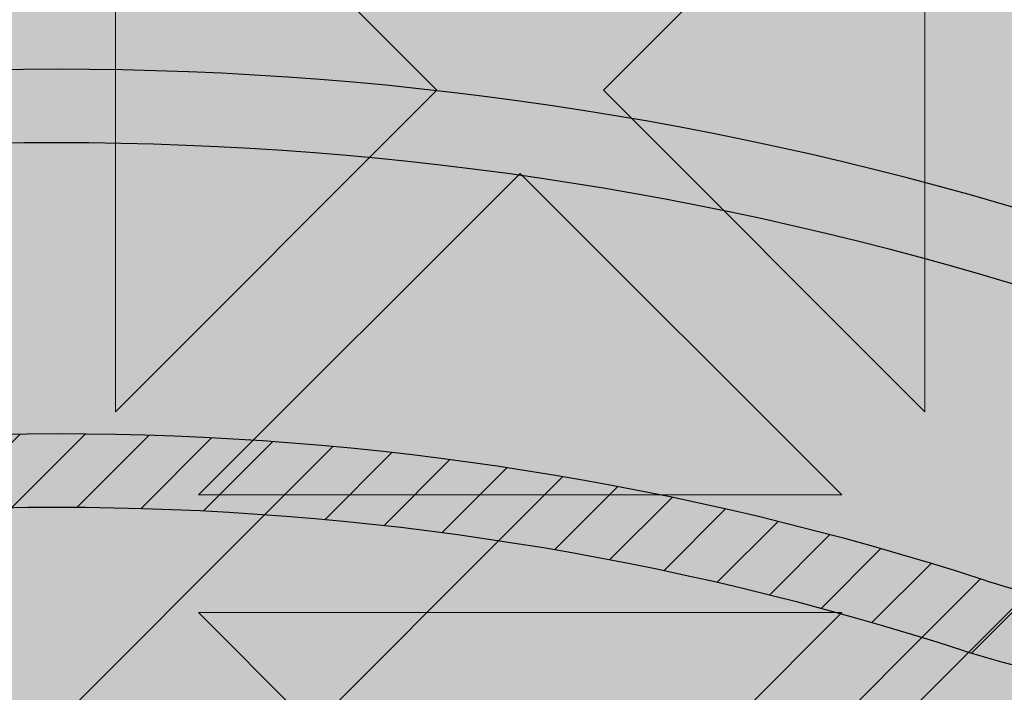
# Model space of a CAD drawing. Units: inches. Extents: x 844 to 2234, y 346 to 1084.
# Tile 20 of 93: x 1122.777 to 1124.911, y 703.603 to 705.06. Entities that reach past the tile are written whole.
import ezdxf

# ---------------------------------------------------------------- set-up
doc = ezdxf.new("R2010")
doc.units = ezdxf.units.IN
doc.header["$MEASUREMENT"] = 0
for name, color, linetype, lineweight in [('A-ANNO-DIMS', 2, 'Continuous', 18), ('furniture', 8, 'Continuous', 18), ('RA-AP-01$0$INT', 35, 'Continuous', 5)]:
    doc.layers.add(name, color=color, linetype=linetype, lineweight=lineweight)
doc.layers.add('RA-AP-01$0$FURN', color=3, linetype='Continuous')
doc.layers.add('RA-AP-01$0$WOOD', color=64, linetype='Continuous')
doc.styles.get("Standard").update_dxf_attribs({"font": 'arial.ttf'})
doc.dimstyles.get("Standard").update_dxf_attribs({"dimtxt": 6, "dimasz": 3, "dimexe": 0.18, "dimexo": 0.0625, "dimgap": 0.09, "dimtad": 0, "dimtih": 1, "dimtoh": 1, "dimdec": 1, "dimzin": 0, "dimdsep": 46, "dimlunit": 3, "dimtxsty": 'Standard', "dimblk": 'ARCHTICK', "dimcen": 0.09, "dimadec": 0, "dimazin": 0, "dimtfac": 1, "dimtdec": 1, "dimtofl": 0, "dimtmove": 0, "dimatfit": 3, "dimfxl": 1, "dimtolj": 1, "dimtzin": 0, "dimarcsym": 0})

# ---------------------------------------------------------------- blocks, each defined once
blk = doc.blocks.new('A$C18D01794')
at = {"layer": 'RA-AP-01$0$INT'}
h = blk.add_hatch(color=256, dxfattribs=at)
h.paths.add_polyline_path([(4.585917135068448, -7.856712009587804), (4.614201406330596, -7.856712009587056), (4.668846067270487, -7.802067348644738), (4.723490728212344, -7.856712009584164), (4.771774999457151, -7.856712009582887), (4.826419660396886, -7.80206734864072), (4.862780050090322, -7.838427738332541), (4.844495778842715, -7.856712009580965), (4.862780050090411, -7.856712009580482), (4.905206456960182, -7.814285602707865), (4.947632863832445, -7.856712009578238), (4.965917135079675, -7.856712009577755), (4.947632863831759, -7.838427738330656), (4.983993253523576, -7.802067348637219), (5.038637914464627, -7.856712009575829), (5.08692218571208, -7.856712009574554), (5.141566846649976, -7.802067348634224), (5.196211507589851, -7.856712009571666), (5.224495778822615, -7.856712009570916), (4.905206456953975, -7.537422687702283)])
h.paths.add_polyline_path([(4.895206456956031, -7.575706958950402), (4.895206456958921, -7.684996280828174), (4.840561796018589, -7.630351619890275)], flags=16)
h.paths.add_polyline_path([(4.915206456955638, -7.575706958949956), (4.969851117895509, -7.630351619887399), (4.915206456957609, -7.684996280827732)], flags=16)
h.paths.add_polyline_path([(4.826419660395175, -7.644493755514321), (4.881064321335613, -7.699138416452331), (4.771774999456703, -7.69913841645522)], flags=16)
h.paths.add_polyline_path([(4.983993253519558, -7.644493755510815), (5.038637914460456, -7.699138416449285), (4.929348592581548, -7.69913841645126)], flags=16)
h.paths.add_polyline_path([(4.881064321336025, -7.719138416452334), (4.826419660397532, -7.773783077393256), (4.771774999457062, -7.719138416455217)], flags=16)
h.paths.add_polyline_path([(4.929348592582019, -7.71913841645126), (5.038637914460982, -7.719138416449284), (4.983993253522945, -7.773783077389749)], flags=16)
h.paths.add_polyline_path([(4.895206456960191, -7.733280552075633), (4.895206456962115, -7.806001331460164), (4.876922185715016, -7.824285602708492), (4.840561796021581, -7.787925213016675)], flags=16)
h.paths.add_polyline_path([(4.915206456958487, -7.733280552075187), (4.969851117899527, -7.787925213013798), (4.933490728206909, -7.824285602708034), (4.9152064569598, -7.806001331461736)], flags=16)
h.paths.add_polyline_path([(4.757632863832376, -7.733280552079264), (4.812277524772842, -7.787925213017304), (4.757632863834348, -7.842569873958233)], flags=16)
h.paths.add_polyline_path([(4.737632863832376, -7.73328055207979), (4.737632863834348, -7.842569873958701), (4.682988202893906, -7.787925213020692)], flags=16)
h.paths.add_polyline_path([(5.05278005008503, -7.733280552072701), (5.052780050087917, -7.842569873951664), (4.998135389146995, -7.787925213013169)], flags=16)
h.paths.add_polyline_path([(5.072780050085024, -7.733280552072333), (5.127424711025931, -7.787925213010806), (5.072780050087916, -7.842569873951244)], flags=16)
h.paths.add_polyline_path([(4.935917135072783, -7.506712009583784), (5.255206456948811, -7.826001331459767), (5.255206456948932, -7.797717060211899), (5.200561796010279, -7.743072399273238), (5.255206456949403, -7.688427738334128), (5.25520645694961, -7.640143467086677), (5.200561796009787, -7.585498806146837), (5.236922185702417, -7.549138416454212), (5.255206456949919, -7.56742268770172), (5.255206456949998, -7.549138416454178), (5.212780050078687, -7.506712009583814), (5.25520645695036, -7.464285602712145), (5.255206456950438, -7.446001331464763), (5.236922185702424, -7.464285602712779), (5.200561796009796, -7.427925213020149), (5.255206456950753, -7.373280552079203), (5.25520645695096, -7.324996280834394), (5.200561796010322, -7.270351619893748), (5.255206456951428, -7.215706958952649), (5.255206456951547, -7.187422687705071)])
h.paths.add_polyline_path([(5.042988202883395, -7.42792521302065), (5.097632863823085, -7.373280552080975), (5.097632863822622, -7.482569873959883)], flags=16)
h.paths.add_polyline_path([(5.028846067259663, -7.442067348644384), (5.083490728198774, -7.496712009583504), (4.974201406321001, -7.496712009583035)], flags=16)
h.paths.add_polyline_path([(5.117632863823087, -7.37328055208089), (5.172277524762331, -7.42792521302015), (5.11763286382262, -7.482569873959851)], flags=16)
h.paths.add_polyline_path([(5.08349072819877, -7.516712009582191), (5.028846067259652, -7.571356670521302), (4.974201406320998, -7.516712009582638)], flags=16)
h.paths.add_polyline_path([(5.131774999446817, -7.35913841645716), (5.186419660386065, -7.413783077396415), (5.241064321325782, -7.359138416456712)], flags=17)
h.paths.add_polyline_path([(5.131774999446228, -7.496712009583703), (5.186419660386065, -7.442067348643883), (5.222780050079488, -7.478427738337313), (5.204495778832781, -7.496712009584014)], flags=16)
h.paths.add_polyline_path([(5.097632863822613, -7.530854145205813), (5.097632863823061, -7.640143467084723), (5.042988202883383, -7.585498806145032)], flags=16)
h.paths.add_polyline_path([(5.131774999446899, -7.339138416457162), (5.241064321325809, -7.339138416456712), (5.186419660386591, -7.284493755517479)], flags=17)
h.paths.add_polyline_path([(5.131774999446226, -7.516712009581999), (5.204495778830767, -7.516712009581702), (5.22278005007868, -7.534996280829206), (5.186419660386049, -7.571356670521828)], flags=16)
h.paths.add_polyline_path([(5.11763286382262, -7.530854145205852), (5.17227752476232, -7.585498806145562), (5.117632863823064, -7.64014346708481)], flags=16)
h.paths.add_polyline_path([(5.186419660386069, -7.599640941770585), (5.241064321325754, -7.654285602710281), (5.131774999446791, -7.654285602709814)], flags=16)
h.paths.add_polyline_path([(5.131774999446872, -7.674285602709813), (5.24106432132578, -7.674285602710282), (5.186419660386554, -7.728930263649504)], flags=16)
h.paths.add_polyline_path([(5.255206456951811, -7.126001331467467), (5.255206456951895, -7.106712009588038), (4.555206456956052, -7.106712009588038), (4.555206456956136, -7.12600133146746), (4.905206456953973, -7.476001331465289)])
h.paths.add_polyline_path([(4.983993253513404, -7.368930263651977), (4.92934859257295, -7.314285602713969), (5.03863791445186, -7.314285602711063)], flags=16)
h.paths.add_polyline_path([(4.969851117889988, -7.383072399276016), (4.915206456952556, -7.437717060215906), (4.915206456949648, -7.328427738338133)], flags=16)
h.paths.add_polyline_path([(4.929348592572535, -7.294285602713971), (4.983993253511019, -7.239640941773039), (5.038637914451496, -7.294285602711065)], flags=16)
h.paths.add_polyline_path([(5.052780050074912, -7.280143467087016), (4.998135389134438, -7.225498806148989), (5.052780050072919, -7.170854145208052)], flags=16)
h.paths.add_polyline_path([(5.07278005007491, -7.280143467086489), (5.072780050072918, -7.170854145207579), (5.127424711013374, -7.225498806145578)], flags=16)
h.paths.add_polyline_path([(4.89520645695295, -7.437717060216355), (4.840561796013067, -7.383072399278919), (4.895206456950961, -7.328427738338582)], flags=16)
h.paths.add_polyline_path([(4.915206456948365, -7.280143467090674), (4.915206456946434, -7.207422687704125), (4.933490728192729, -7.18913841645701), (4.969851117886972, -7.225498806149623)], flags=16)
h.paths.add_polyline_path([(4.881064321327021, -7.314285602715054), (4.82641966038902, -7.368930263655506), (4.771774999448108, -7.314285602717047)], flags=16)
h.paths.add_polyline_path([(4.895206456950073, -7.280143467091125), (4.840561796009022, -7.225498806152518), (4.876922185700835, -7.18913841645908), (4.895206456948749, -7.207422687706589)], flags=16)
h.paths.add_polyline_path([(4.983993253510392, -7.211356670525576), (4.947632863816944, -7.174996280833758), (4.965917135064043, -7.156712009585847), (5.038637914448995, -7.156712009584522)], flags=16)
h.paths.add_polyline_path([(4.881064321326543, -7.294285602715056), (4.771774999447578, -7.294285602717046), (4.826419660385607, -7.239640941776569)], flags=16)
h.paths.add_polyline_path([(4.905206456946447, -7.19913841645844), (4.862780050074785, -7.156712009587725), (4.947632863816685, -7.156712009586302)], flags=16)
h.paths.add_polyline_path([(5.14156684663679, -7.211356670521528), (5.086922185696452, -7.156712009583639), (5.196211507574223, -7.156712009581651)], flags=16)
h.paths.add_polyline_path([(4.8264196603837, -7.211356670529104), (4.771774999442643, -7.156712009590501), (4.8444957788276, -7.156712009588568), (4.862780050075511, -7.17499628083566)], flags=16)
h.paths.add_polyline_path([(4.812277524760289, -7.225498806153156), (4.757632863822258, -7.28014346709363), (4.757632863819352, -7.170854145214669)], flags=16)
h.paths.add_polyline_path([(4.73763286382226, -7.280143467093997), (4.682988202881349, -7.22549880615554), (4.737632863819352, -7.170854145215086)], flags=16)
h.paths.add_polyline_path([(4.723490728195188, -7.156712009591787), (4.668846067257299, -7.211356670532127), (4.614201406317417, -7.156712009594693)], flags=16)
h.paths.add_polyline_path([(4.597632863829262, -7.506712009583814), (4.555206456957951, -7.54913841645418), (4.555206456958029, -7.56742268770172), (4.573490728205535, -7.549138416454212), (4.609851117898167, -7.585498806146839), (4.555206456958338, -7.640143467086675), (4.555206456958546, -7.688427738334125), (4.60985111789767, -7.743072399273238), (4.555206456959015, -7.797717060211899), (4.555206456959138, -7.826001331459767), (4.874495778835167, -7.506712009583786), (4.5552064569564, -7.187422687705062), (4.555206456956523, -7.215706958952644), (4.609851117897629, -7.270351619893746), (4.555206456956988, -7.324996280834396), (4.555206456957198, -7.373280552079195), (4.609851117898153, -7.427925213020147), (4.573490728205528, -7.464285602712779), (4.555206456957507, -7.446001331464756), (4.555206456957585, -7.464285602712143)])
h.paths.add_polyline_path([(4.712780050085332, -7.482569873959882), (4.712780050084863, -7.373280552080972), (4.767424711024555, -7.42792521302065)], flags=16)
h.paths.add_polyline_path([(4.726922185709173, -7.496712009583504), (4.781566846648288, -7.442067348644384), (4.836211507586949, -7.496712009583033)], flags=16)
h.paths.add_polyline_path([(4.692780050085327, -7.482569873959851), (4.638135389145619, -7.427925213020149), (4.692780050084865, -7.373280552080892)], flags=16)
h.paths.add_polyline_path([(4.726922185709182, -7.516712009582191), (4.836211507586949, -7.51671200958264), (4.7815668466483, -7.571356670521304)], flags=16)
h.paths.add_polyline_path([(4.678637914461726, -7.496712009583706), (4.605917135075169, -7.496712009584014), (4.587632863828464, -7.478427738337311), (4.623993253521887, -7.442067348643881)], flags=16)
h.paths.add_polyline_path([(4.712780050085336, -7.530854145205816), (4.767424711024568, -7.585498806145034), (4.71278005008489, -7.640143467084724)], flags=16)
h.paths.add_polyline_path([(4.678637914461726, -7.516712009582001), (4.623993253521899, -7.571356670521829), (4.587632863829271, -7.534996280829206), (4.605917135077185, -7.5167120095817)], flags=16)
h.paths.add_polyline_path([(4.692780050085336, -7.530854145205848), (4.692780050084889, -7.64014346708481), (4.638135389145632, -7.585498806145562)], flags=16)
h.paths.add_polyline_path([(4.623993253521885, -7.413783077396415), (4.678637914461131, -7.359138416457161), (4.56934859258217, -7.359138416456712)], flags=17)
h.paths.add_polyline_path([(4.623993253521901, -7.599640941770568), (4.678637914461158, -7.654285602709814), (4.569348592582195, -7.654285602710281)], flags=16)
h.paths.add_polyline_path([(4.678637914461051, -7.339138416457162), (4.623993253521361, -7.284493755517479), (4.569348592582143, -7.339138416456712)], flags=17)
h.paths.add_polyline_path([(4.678637914461076, -7.674285602709813), (4.623993253521399, -7.728930263649504), (4.569348592582167, -7.674285602710281)], flags=16)
h = blk.add_hatch(color=256, dxfattribs=at)
h.paths.add_polyline_path([(4.905206456954232, -7.537422687702028), (4.874495778835232, -7.506712009583718), (4.555206456959138, -7.826001331459766), (4.555206456959269, -7.856712009588616), (4.585917135068449, -7.856712009587804)])
h.paths.add_polyline_path([(4.935917135072152, -7.506712009583152), (4.905206456953497, -7.537422687701806), (5.224495778822614, -7.856712009570917), (5.255206456948681, -7.856712009570104), (5.255206456948813, -7.826001331459768)])
h.paths.add_polyline_path([(5.255206456951549, -7.18742268770507), (5.255206456951813, -7.126001331467461), (4.905206456953563, -7.476001331465701), (4.935917135072559, -7.506712009584006)])
h.paths.add_polyline_path([(4.874495778835167, -7.506712009583785), (4.905206456953818, -7.476001331465132), (4.555206456956135, -7.126001331467458), (4.555206456956399, -7.187422687705064)])
h = blk.add_hatch(color=256, dxfattribs=at)
h.paths.add_polyline_path([(4.969851117891331, -7.630351619889621), (4.915206456952669, -7.575706958950966), (4.915206456952222, -7.684996280828739)])
h.paths.add_polyline_path([(4.895206456953064, -7.575706958950968), (4.840561796014413, -7.630351619889628), (4.895206456953533, -7.684996280828741)])
h.paths.add_polyline_path([(4.826419660390684, -7.644493755513362), (4.771774999451003, -7.699138416453052), (4.881064321329913, -7.699138416452587)])
h.paths.add_polyline_path([(4.881064321329884, -7.719138416452585), (4.771774999450921, -7.719138416453052), (4.82641966039018, -7.773783077392298)])
h.paths.add_polyline_path([(4.895206456953734, -7.733280552076196), (4.840561796013912, -7.787925213016031), (4.876922185707337, -7.824285602709455), (4.895206456954043, -7.806001331462747)])
h.paths.add_polyline_path([(4.862780050082808, -7.838427738332388), (4.826419660390178, -7.802067348639763), (4.771774999450351, -7.856712009579595), (4.844495778835303, -7.856712009579895)])
h.paths.add_polyline_path([(4.812277524766446, -7.787925213016036), (4.757632863827191, -7.733280552076788), (4.757632863826741, -7.842569873955747)])
h.paths.add_polyline_path([(4.737632863827191, -7.733280552076863), (4.682988202887508, -7.787925213016558), (4.737632863826743, -7.842569873955778)])
h.paths.add_polyline_path([(4.668846067263777, -7.802067348640287), (4.614201406325123, -7.856712009578949), (4.723490728202894, -7.856712009579402)])
h.paths.add_polyline_path([(4.905206456953846, -7.814285602708654), (4.862780050082654, -7.856712009579847), (4.947632863824561, -7.85671200958032)])
h.paths.add_polyline_path([(4.915206456952028, -7.733280552076195), (4.91520645695173, -7.806001331460731), (4.933490728199234, -7.824285602708648), (4.96985111789186, -7.787925213016022)])
h.paths.add_polyline_path([(5.038637914454841, -7.719138416453029), (4.929348592575874, -7.71913841645258), (4.983993253515593, -7.773783077392289)])
h.paths.add_polyline_path([(4.983993253515065, -7.644493755513352), (4.929348592575849, -7.699138416452582), (5.038637914454755, -7.699138416453031)])
h.paths.add_polyline_path([(5.052780050079843, -7.73328055207676), (4.998135389140595, -7.787925213016018), (5.052780050080309, -7.842569873955721)])
h.paths.add_polyline_path([(4.983993253516868, -7.802067348639752), (4.947632863824241, -7.838427738332383), (4.965917135071747, -7.856712009579888), (5.038637914456701, -7.856712009579572)])
h.paths.add_polyline_path([(5.127424711019533, -7.787925213016519), (5.072780050079843, -7.733280552076838), (5.07278005008031, -7.842569873955751)])
h.paths.add_polyline_path([(5.141566846643269, -7.802067348640248), (5.086922185704154, -7.85671200957937), (5.196211507581929, -7.856712009578901)])
for p, q in [((4.905206456953975, -7.537422687702283), (5.224495778822613, -7.856712009570916)), ((4.929348592581546, -7.69913841645126), (4.983993253519556, -7.644493755510815)), ((4.983993253519558, -7.644493755510817), (5.038637914460456, -7.699138416449285)), ((5.038637914460456, -7.699138416449285), (4.929348592581546, -7.69913841645126)), ((5.038637914460983, -7.719138416449284), (4.92934859258202, -7.71913841645126)), ((4.92934859258202, -7.71913841645126), (4.983993253522945, -7.773783077389751)), ((5.038637914460983, -7.719138416449284), (4.983993253522945, -7.773783077389751)), ((4.9152064569598, -7.806001331460137), (4.915206456958485, -7.733280552075186)), ((4.915206456958485, -7.733280552075186), (4.969851117899529, -7.787925213013799)), ((5.052780050085028, -7.733280552072701), (4.998135389146995, -7.787925213013169)), ((5.052780050085028, -7.733280552072701), (5.052780050087917, -7.842569873951664)), ((4.969851117899529, -7.787925213013798), (4.93349072820771, -7.824285602707234)), ((5.052780050087917, -7.842569873951664), (4.998135389146995, -7.787925213013169))]:
    blk.add_line(p, q, dxfattribs=at)
blk = doc.blocks.new('A$C32926AE1')
at = {"layer": 'RA-AP-01$0$WOOD'}
h = blk.add_hatch(color=256, dxfattribs=at)
h.dxf.hatch_style = 1
h.paths.add_polyline_path([(5.157430609644524, 4.573483066760929, -0.1009492694046607), (5.155401577623758, 4.593365984175333, -0.1842662638101597), (5.172249623284174, 4.638795604568598, 0.2056608120311276), (5.179560981299304, 4.661316324430096, 0.3614336704623542), (5.134352340494423, 4.706524965234944, 0.2056608120311297), (5.111831620632933, 4.699213607219793, -0.1842662638101113), (5.066402000239693, 4.682365561559342, -0.1055311479399994), (5.045656153913092, 4.68467289944697, 0.1567636581983829), (4.763886414745334, 4.684672899446966, -0.1055311479399895), (4.743140568418733, 4.68236556155934, -0.1842662638100833), (4.6977109480255, 4.69921360721979, 0.2056608120302612), (4.675190228164109, 4.706524965234949, 0.3614336704708441), (4.629981587358889, 4.66131632442871, 0.2056608120245944), (4.637292945374126, 4.638795604567974, -0.1842662638101024), (4.654140991034615, 4.59336598417475, -0.1009492694055169), (4.652111959013835, 4.573483066760181, 0.021410119221476), (4.629748025606143, 4.156712009541676, 0.0214101192214795), (4.652111959013809, 3.739940952323101, -0.1009492694059586), (4.654140991034615, 3.720058034908448, -0.1842662638100975), (4.637292945374126, 3.674628414515226, 0.2056608120245705), (4.629981587358889, 3.652107694654492, 0.3614336704708879), (4.675190228164113, 3.606899053848249, 0.2056608120302384), (4.697710948025501, 3.614210411863408, -0.1842662638100995), (4.743140568418738, 3.63105845752386, -0.1055311479402541), (4.763886414745388, 3.628751119636215, 0.1567636581983776), (5.045656153913137, 3.628751119636244, -0.1055311479397538), (5.066402000239692, 3.631058457523857, -0.1842662638101067), (5.111831620632931, 3.614210411863407, 0.2056608120310924), (5.134352340494417, 3.606899053848256, 0.3614336704624001), (5.179560981299307, 3.652107694653103, 0.2056608120311314), (5.172249623284175, 3.6746284145146, -0.1842662638101402), (5.155401577623758, 3.72005803490786, -0.1009492694051366), (5.15743060964455, 3.739940952322354, 0.0214101192215073), (5.179794543052287, 4.156712009541468, 0.0214101192215252)])
h.paths.add_polyline_path([(4.639748609479751, 4.156712009541513, 0.0213537860821624), (4.661970494867118, 3.741887061152232, -0.094075836301374), (4.664143710413708, 3.7196126951003, -0.1824818158568985), (4.644813765429836, 3.668037719127816, 0.2056608120245319), (4.639939526753007, 3.653023905887301, 0.3614336704710246), (4.676106439397173, 3.616856993242342, 0.2056608120302234), (4.691120252638095, 3.621731231919122, -0.1824818158602558), (4.742695228611606, 3.641061176902986, -0.1029891339458722), (4.766991894714349, 3.638256818950944, 0.156709409989566), (5.042550673941472, 3.638256818950105, -0.102989133958497), (5.066847340047078, 3.641061176902949, -0.1824818158594995), (5.118422316020358, 3.621731231919103, 0.2056608120311416), (5.133436129261316, 3.616856993242346, 0.3614336704621468), (5.169603041905217, 3.653023905886178, 0.2056608120310986), (5.164728803228477, 3.668037719127177, -0.1824818158565612), (5.145398858244737, 3.719612695099578, -0.0940758363009313), (5.147572073791232, 3.741887061151398, 0.0213537860822023), (5.169793959178681, 4.156712009541451, 0.0213537860822226), (5.147572073791203, 4.571536957931898, -0.0940758363005034), (5.145398858244737, 4.59381132398362, -0.1824818158565587), (5.164728803228476, 4.645386299956021, 0.2056608120311045), (5.169603041905216, 4.66040011319702, 0.3614336704621845), (5.133436129261313, 4.696567025840856, 0.2056608120310773), (5.118422316020359, 4.691692787164098, -0.182481815859508), (5.066847340047078, 4.67236284218025, -0.1029891339584606), (5.04255067394148, 4.675167200133092, 0.156709409989566), (4.766991894714357, 4.675167200132257, -0.1029891339458842), (4.742695228611611, 4.672362842180213, -0.1824818158602725), (4.691120252638095, 4.691692787164077, 0.2056608120302152), (4.676106439397174, 4.696567025840858, 0.3614336704710363), (4.639939526753005, 4.660400113195899, 0.2056608120245495), (4.644813765429837, 4.645386299955384, -0.1824818158568934), (4.664143710413708, 4.593811323982902, -0.0940758363009187), (4.661970494867149, 4.571536957931074, 0.021353786082177)], flags=16)
h.paths.add_polyline_path([(5.129794543052235, 4.432167055276933, -0.0141661062790638), (5.130152669293814, 4.156927903047693, -0.0141661062790647), (5.129794543052234, 3.881688750818433, -0.0785247771143638), (5.10979738006795, 3.755143611847103, 0.0945969212073497), (5.105408519571111, 3.717898134952927, 0.1043170707844957), (5.116074640131521, 3.670385395016088, 0.1043170707864965), (5.068561900193738, 3.681051515576561, 0.09459692119553), (5.031316423304057, 3.676662655080835, -0.1580239521427272), (4.778226145355827, 3.676662655080367, 0.0945969211986668), (4.740980668464973, 3.681051515576592, 0.1043170707882822), (4.693467928526415, 3.670385395015844, 0.1043170707867916), (4.704134049087309, 3.717898134953662, 0.0945969211972894), (4.69974518859162, 3.755143611844042, -0.0785247771163196), (4.679748025606343, 3.881688750818406, -0.0141661062790663), (4.679389899364763, 4.156927903047693, -0.0141661062790672), (4.679748025606343, 4.432167055276998, -0.0785247771163064), (4.699745188591625, 4.55871219425134, 0.094596921197333), (4.704134049087308, 4.595957671141738, 0.1043170707867205), (4.693467928526416, 4.643470411079523, 0.1043170707882628), (4.740980668464965, 4.632804290518776, 0.0945969211988114), (4.778226145355874, 4.637193151015016, -0.158023952142669), (5.031316423304015, 4.637193151014546, 0.0945969211956361), (5.068561900193736, 4.632804290518806, 0.1043170707864979), (5.11607464013152, 4.643470411079278, 0.1043170707844617), (5.105408519571112, 4.595957671142455, 0.0945969212074597), (5.109797380067959, 4.558712194248236, -0.0785247771143467)], flags=0)
h.paths.add_polyline_path([(5.119794532311105, 4.432259799204851, -0.0142000800617244), (5.120156169157484, 4.156927903047701, -0.0142000800617277), (5.119794532311105, 3.881596006890482, -0.0784894509520253), (5.100273383573699, 3.758192358677797, 0.0940138827242913), (5.095413455884425, 3.717477693979438, 0.0606271852308753), (5.099615656341024, 3.686844378806616, 0.0606271852322524), (5.068982341167493, 3.691046579263239, 0.0940138827010453), (5.028267676478798, 3.686186651576848, -0.1580706864508061), (4.781274892180912, 3.686186651576435, 0.0940138827026903), (4.740560227491556, 3.691046579263279, 0.0606271852339895), (4.709926912317155, 3.686844378806508, 0.0606271852329405), (4.714129112773991, 3.717477693980356, 0.094013882701304), (4.709269185087677, 3.758192358669163, -0.0784894509577193), (4.689748036347473, 3.881596006890469, -0.014200080061729), (4.689386399501094, 4.156927903047709, -0.0142000800617217), (4.689748036347473, 4.432259799204808, -0.078489450957724), (4.709269185087651, 4.555663447426125, 0.0940138827014585), (4.714129112773992, 4.596378112114996, 0.0606271852329731), (4.709926912317154, 4.62701142728886, 0.0606271852340196), (4.74056022749157, 4.622809226832087, 0.0940138827024997), (4.781274892180847, 4.627669154518912, -0.1580706864508359), (5.028267676478777, 4.627669154518526, 0.0940138827010946), (5.068982341167492, 4.622809226832129, 0.060627185232254), (5.099615656341024, 4.627011427288751, 0.0606271852308727), (5.095413455884425, 4.59637811211593, 0.0940138827241088), (5.100273383573675, 4.555663447417647, -0.0784894509520978)], flags=0)
h.paths.add_polyline_path([(5.06978912287499, 4.430218106756144, -0.014241683694547), (5.070173729147532, 4.156927903047672, -0.0142416836945458), (5.06978912287499, 3.883637699339223, -0.0800609523125196), (5.052662118612511, 3.773463122773442, 0.0526421978001116), (5.04590916754064, 3.740550867606997, 0.0526421977992423), (5.012996912374707, 3.73379791653534, -0.1583028414718258), (4.796545656286308, 3.73379791653451, 0.0526421978034211), (4.763633401117837, 3.740550867607021, 0.0526421978018622), (4.756880450045755, 3.773463122774558, -0.0800609523117106), (4.739753445783639, 3.883637699339268, -0.0142416836945435), (4.739368839511098, 4.156927903047671, -0.0142416836945477), (4.739753445783639, 4.430218106756155, -0.0800609523116345), (4.75688045004574, 4.540392683320762, 0.052642197801941), (4.763633401117837, 4.573304938488346, 0.0526421978035071), (4.796545656286361, 4.580057889560873, -0.1583028414717561), (5.012996912374669, 4.580057889560039, 0.0526421977993048), (5.04590916754064, 4.57330493848837, 0.0526421978002057), (5.052662118612529, 4.540392683321868, -0.080060952312477)], flags=0)
h.paths.add_polyline_path([(5.049789715110557, 4.43038092723357, -0.0143097550741839), (5.05018085590259, 4.156927903047715, -0.0143097550741854), (5.049789715110558, 3.883474878861827, -0.0800685599149176), (5.03362098255317, 3.779581877367999, 0.0306258898956367), (5.028241146483733, 3.758218888663947, 0.0306258898977031), (5.006878157778253, 3.75283905259408, -0.1583983521624096), (4.802664410878162, 3.752839052594731, 0.0306258898946014), (4.781301422174808, 3.758218888663924, 0.0306258898967912), (4.775921586105202, 3.779581877368794, -0.080068559914251), (4.759752853548071, 3.883474878861786, -0.0143097550741854), (4.759361712756037, 4.156927903047671, -0.0143097550741854), (4.759752853548071, 4.430380927233557, -0.0800685599142479), (4.775921586105193, 4.534273928726546, 0.0306258898968306), (4.781301422174808, 4.555636917431444, 0.0306258898945754), (4.802664410878143, 4.561016753500631, -0.1583983521624168), (5.006878157778244, 4.561016753501291, 0.0306258898977177), (5.028241146483733, 4.555636917431421, 0.0306258898958182), (5.03362098255321, 4.534273928727244, -0.080068559914796)], flags=0)
h.paths.add_polyline_path([(4.999766070382627, 4.428171244713864, -0.0143443147609634), (5.000198441819402, 4.156927903047689, -0.0143443147609612), (4.999766070382627, 3.885684561381556, -0.0784641635803329), (4.987356730658798, 3.799103304488872, -0.1506053783831347), (4.822185837999821, 3.79910330448882, -0.0784641635803318), (4.809776498276007, 3.885684561381509, -0.014344314760963), (4.809344126839227, 4.156927903047677, -0.0143443147609645), (4.809776498276007, 4.428171244713873, -0.0784641635803192), (4.822185837999822, 4.514752501606549, -0.1506053783831338), (4.987356730658798, 4.514752501606494, -0.078464163580285)], flags=0)
h.paths.add_polyline_path([(4.979755254238824, 4.42764379880488, -0.0143772539198268), (4.980205517789977, 4.156927903047693, -0.0143772539198275), (4.979755254238824, 3.886212007290489, -0.0689242507424422), (4.971183264704897, 3.815276770442801, -0.1296645318904179), (4.838359303953726, 3.815276770442746, -0.0689242507424186), (4.829787314419809, 3.886212007290419, -0.0143772539198292), (4.829337050868653, 4.156927903047653, -0.0143772539198325), (4.829787314419809, 4.427643798804946, -0.0689242507424211), (4.838359303953725, 4.498579035652621, -0.1296645318904187), (4.971183264704897, 4.498579035652565, -0.0689242507424401)], flags=0)
h = blk.add_hatch(color=256, dxfattribs=at)
h.dxf.hatch_style = 1
h.paths.add_polyline_path([(5.145398858244737, 4.59381132398362, -0.1824818158565616), (5.164728803228476, 4.645386299956021, 0.2056608120311045), (5.169603041905216, 4.66040011319702, 0.3614336704621845), (5.133436129261313, 4.696567025840856, 0.2056608120310773), (5.118422316020359, 4.691692787164098, -0.182481815859508), (5.066847340047078, 4.67236284218025, -0.1029891339584606), (5.04255067394148, 4.675167200133092, 0.156709409989566), (4.766991894714357, 4.675167200132257, -0.1029891339458842), (4.742695228611611, 4.672362842180213, -0.1824818158602725), (4.691120252638095, 4.691692787164077, 0.2056608120302152), (4.676106439397174, 4.696567025840858, 0.3614336704710363), (4.639939526753005, 4.660400113195899, 0.2056608120245495), (4.644813765429837, 4.645386299955384, -0.1824818158568934), (4.664143710413708, 4.593811323982902, -0.0940758363009187), (4.661970494867149, 4.571536957931074, 0.0213537860821772), (4.639748609479751, 4.156712009541507, 0.0213537860821625), (4.661970494867119, 3.741887061152226, -0.0940758363013071), (4.664143710413708, 3.719612695100309, -0.1824818158569294), (4.644813765429836, 3.668037719127816, 0.2056608120245319), (4.639939526753007, 3.653023905887301, 0.3614336704710246), (4.676106439397173, 3.616856993242342, 0.2056608120302234), (4.691120252638095, 3.621731231919122, -0.1824818158602558), (4.742695228611606, 3.641061176902986, -0.1029891339458722), (4.766991894714349, 3.638256818950944, 0.156709409989566), (5.042550673941472, 3.638256818950105, -0.102989133958497), (5.066847340047078, 3.641061176902949, -0.1824818158594995), (5.118422316020358, 3.621731231919103, 0.2056608120311416), (5.133436129261316, 3.616856993242346, 0.3614336704621468), (5.169603041905217, 3.653023905886178, 0.2056608120310986), (5.164728803228477, 3.668037719127177, -0.1824818158565612), (5.145398858244737, 3.719612695099578, -0.0940758363009313), (5.147572073791232, 3.741887061151398, 0.0213537860822023), (5.169793959178681, 4.156712009541451, 0.0213537860822226), (5.147572073791203, 4.571536957931898, -0.0940758363004996)])
h.paths.add_polyline_path([(5.109797380067958, 4.55871219424824, -0.0785247771143472), (5.129794543052234, 4.432167055276936, -0.0141661062790644), (5.130152669293814, 4.156927903047685, -0.014166106279066), (5.129794543052234, 3.881688750818401, -0.0785247771143517), (5.109797380067946, 3.755143611847092, 0.0945969212073132), (5.105408519571111, 3.717898134952929, 0.1043170707844995), (5.116074640131521, 3.670385395016088, 0.1043170707864965), (5.068561900193738, 3.681051515576561, 0.09459692119553), (5.031316423304057, 3.676662655080835, -0.1580239521427272), (4.778226145355827, 3.676662655080367, 0.0945969211986668), (4.740980668464973, 3.681051515576592, 0.1043170707882822), (4.693467928526415, 3.670385395015844, 0.1043170707867916), (4.704134049087309, 3.717898134953662, 0.0945969211972894), (4.69974518859162, 3.755143611844042, -0.0785247771163196), (4.679748025606343, 3.881688750818406, -0.0141661062790663), (4.679389899364763, 4.156927903047693, -0.0141661062790672), (4.679748025606343, 4.432167055276998, -0.0785247771163064), (4.699745188591625, 4.55871219425134, 0.094596921197333), (4.704134049087308, 4.595957671141738, 0.1043170707867205), (4.693467928526416, 4.643470411079523, 0.1043170707882628), (4.740980668464965, 4.632804290518776, 0.0945969211988114), (4.778226145355874, 4.637193151015016, -0.158023952142669), (5.031316423304015, 4.637193151014546, 0.0945969211956361), (5.068561900193736, 4.632804290518806, 0.1043170707864979), (5.11607464013152, 4.643470411079278, 0.1043170707844617), (5.105408519571112, 4.595957671142455, 0.0945969212074504)], flags=16)
h.paths.add_polyline_path([(5.100273383573655, 4.55566344741771, -0.0784894509521388), (5.119794532311105, 4.432259799204852, -0.0142000800617252), (5.120156169157484, 4.156927903047686, -0.014200080061726), (5.119794532311105, 3.881596006890502, -0.0784894509520446), (5.100273383573696, 3.758192358677786, 0.0940138827242721), (5.095413455884425, 3.717477693979436, 0.0606271852308692), (5.099615656341024, 3.686844378806616, 0.0606271852322522), (5.068982341167493, 3.691046579263239, 0.0940138827010453), (5.028267676478798, 3.686186651576848, -0.1580706864508061), (4.781274892180912, 3.686186651576435, 0.0940138827026903), (4.740560227491556, 3.691046579263279, 0.0606271852339895), (4.709926912317155, 3.686844378806508, 0.0606271852329405), (4.714129112773991, 3.717477693980356, 0.094013882701304), (4.709269185087677, 3.758192358669163, -0.0784894509577193), (4.689748036347473, 3.881596006890469, -0.014200080061729), (4.689386399501094, 4.156927903047709, -0.0142000800617217), (4.689748036347473, 4.432259799204808, -0.078489450957724), (4.709269185087651, 4.555663447426125, 0.0940138827014585), (4.714129112773992, 4.596378112114996, 0.0606271852329731), (4.709926912317154, 4.62701142728886, 0.0606271852340196), (4.74056022749157, 4.622809226832087, 0.0940138827024997), (4.781274892180847, 4.627669154518912, -0.1580706864508359), (5.028267676478777, 4.627669154518526, 0.0940138827010946), (5.068982341167492, 4.622809226832129, 0.060627185232254), (5.099615656341024, 4.627011427288751, 0.0606271852308727), (5.095413455884425, 4.59637811211593, 0.094013882723957)], flags=0)
h.paths.add_polyline_path([(5.04590916754064, 4.57330493848837, 0.0526421978002057), (5.052662118612529, 4.540392683321868, -0.0800609523124783), (5.06978912287499, 4.430218106756142, -0.0142416836945469), (5.070173729147532, 4.156927903047672, -0.0142416836945458), (5.06978912287499, 3.883637699339223, -0.0800609523125196), (5.052662118612511, 3.773463122773442, 0.0526421978001116), (5.04590916754064, 3.740550867606997, 0.0526421977992423), (5.012996912374707, 3.73379791653534, -0.1583028414718258), (4.796545656286308, 3.73379791653451, 0.0526421978034211), (4.763633401117837, 3.740550867607021, 0.0526421978018622), (4.756880450045755, 3.773463122774558, -0.0800609523117106), (4.739753445783639, 3.883637699339268, -0.0142416836945435), (4.739368839511098, 4.156927903047671, -0.0142416836945477), (4.739753445783639, 4.430218106756155, -0.0800609523116345), (4.75688045004574, 4.540392683320762, 0.052642197801941), (4.763633401117837, 4.573304938488346, 0.0526421978035071), (4.796545656286361, 4.580057889560873, -0.1583028414717561), (5.012996912374669, 4.580057889560039, 0.0526421977993048)], flags=0)
h.paths.add_polyline_path([(5.028241146483733, 4.555636917431422, 0.0306258898956949), (5.033620982553182, 4.534273928727329, -0.0800685599148649), (5.049789715110557, 4.430380927233569, -0.0143097550741839), (5.05018085590259, 4.156927903047715, -0.0143097550741854), (5.049789715110558, 3.883474878861827, -0.0800685599149176), (5.03362098255317, 3.779581877367999, 0.0306258898956367), (5.028241146483733, 3.758218888663947, 0.0306258898977031), (5.006878157778253, 3.75283905259408, -0.1583983521624096), (4.802664410878162, 3.752839052594731, 0.0306258898946014), (4.781301422174808, 3.758218888663924, 0.0306258898967912), (4.775921586105202, 3.779581877368794, -0.080068559914251), (4.759752853548071, 3.883474878861786, -0.0143097550741854), (4.759361712756037, 4.156927903047671, -0.0143097550741854), (4.759752853548071, 4.430380927233557, -0.0800685599142479), (4.775921586105193, 4.534273928726546, 0.0306258898968306), (4.781301422174808, 4.555636917431444, 0.0306258898945754), (4.802664410878143, 4.561016753500631, -0.1583983521624168), (5.006878157778244, 4.561016753501291, 0.0306258898977174)], flags=0)
h.paths.add_polyline_path([(4.987356730658798, 4.514752501606494, -0.0784641635803018), (4.999766070382627, 4.428171244713845, -0.0143443147609637), (5.000198441819402, 4.156927903047665, -0.0143443147609622), (4.999766070382628, 3.885684561381514, -0.0784641635802952), (4.987356730658797, 3.799103304488872, -0.1506053783831338), (4.822185837999821, 3.799103304488819, -0.0784641635803342), (4.809776498276007, 3.885684561381512, -0.0143443147609628), (4.809344126839227, 4.156927903047676, -0.0143443147609646), (4.809776498276007, 4.428171244713873, -0.0784641635803192), (4.822185837999822, 4.514752501606549, -0.1506053783831338)], flags=0)
h.paths.add_polyline_path([(4.971183264704897, 4.498579035652566, -0.0689242507424384), (4.979755254238824, 4.427643798804883, -0.0143772539198276), (4.980205517789977, 4.15692790304768, -0.0143772539198258), (4.979755254238823, 3.88621200729051, -0.0689242507424628), (4.971183264704897, 3.815276770442801, -0.129664531890417), (4.838359303953726, 3.815276770442746, -0.0689242507424186), (4.829787314419809, 3.886212007290419, -0.0143772539198292), (4.829337050868653, 4.156927903047653, -0.0143772539198325), (4.829787314419809, 4.427643798804946, -0.0689242507424211), (4.838359303953725, 4.498579035652621, -0.1296645318904187)], flags=0)
h = blk.add_hatch(dxfattribs=at)
h.set_pattern_fill('ANSI31', color=256, scale=0.05, style=0)
h.set_pattern_definition([(45, (0, 0), (-0.0044194173824159, 0.0044194173824159), [])])
h.paths.add_polyline_path([(5.130152669293814, 4.156927903047704, 0.0141661062790657), (5.129794543052234, 4.432167055276982, 0.0777827904001433), (5.110168979996553, 4.557559993161921, -0.0976515123401879), (5.105408519571111, 4.595957671142454, -0.1043170707844687), (5.116074640131522, 4.64347041107928), (5.099615656341024, 4.627011427288751, 0.0606271852308727), (5.095413455884425, 4.59637811211593, 0.0940138827241088), (5.100273383573675, 4.555663447417647, -0.0784894509520972), (5.119794532311105, 4.432259799204852, -0.0142000800617252), (5.120156169157484, 4.156927903047686, -0.014200080061726), (5.119794532311105, 3.881596006890502, -0.0784894509520446), (5.100273383573696, 3.758192358677786, 0.0940138827242721), (5.095413455884425, 3.717477693979436, 0.0606271852308692), (5.099615656341024, 3.686844378806616), (5.116074640131519, 3.67038539501609, -0.1043170707844594), (5.105408519571112, 3.717898134952912, -0.0976515123401594), (5.11016897999655, 3.756295812933435, 0.0777827904001654), (5.129794543052234, 3.881688750818409, 0.0141661062790665)])
h.paths.add_polyline_path([(5.030164222210597, 3.676291055149937, -0.0976515123472002), (5.068561900193739, 3.681051515576561, -0.1043170707864927), (5.116074640131521, 3.670385395016088), (5.099615656341024, 3.686844378806616, 0.0606271852322522), (5.068982341167493, 3.691046579263239, 0.0940138827010453), (5.028267676478798, 3.686186651576848, -0.1580706864508061), (4.781274892180912, 3.686186651576435, 0.0940138827026903), (4.740560227491556, 3.691046579263279, 0.0606271852339913), (4.709926912317154, 3.686844378806508), (4.693467928526416, 3.670385395015845, -0.1043170707882796), (4.740980668464973, 3.681051515576592, -0.0976515123427246), (4.779378346446416, 3.676291055150394, 0.156512506893803)])
h.paths.add_polyline_path([(4.689748036347473, 3.881596006890472, -0.014200080061729), (4.689386399501094, 4.156927903047712, -0.0142000800617195), (4.689748036347473, 4.432259799204768, -0.078489450957742), (4.709269185087648, 4.555663447426114, 0.0940138827014821), (4.714129112773992, 4.596378112114995, 0.0606271852329748), (4.709926912317154, 4.62701142728886), (4.693467928526414, 4.643470411079524, -0.1043170707867939), (4.704134049087309, 4.595957671141706, -0.09765151234893), (4.699373588660725, 4.557559993157876, 0.0777827903975372), (4.679748025606343, 4.432167055276987, 0.0141661062790675), (4.679389899364763, 4.156927903047675, 0.0141661062790641), (4.679748025606343, 3.88168875081843, 0.0777827903975637), (4.699373588660724, 3.756295812937497, -0.0976515123490278), (4.704134049087308, 3.717898134953629, -0.1043170707867196), (4.693467928526416, 3.670385395015845), (4.709926912317155, 3.686844378806508, 0.0606271852329413), (4.714129112773991, 3.717477693980357, 0.0940138827013084), (4.709269185087676, 3.758192358669166, -0.0784894509577192)])
h.paths.add_polyline_path([(4.779378346446434, 4.63756475094498, -0.0976515123427943), (4.740980668464964, 4.632804290518776, -0.1043170707882609), (4.693467928526416, 4.643470411079523), (4.709926912317154, 4.62701142728886, 0.0606271852340196), (4.74056022749157, 4.622809226832087, 0.0940138827024997), (4.781274892180847, 4.627669154518912, -0.1580706864508359), (5.028267676478777, 4.627669154518526, 0.0940138827010946), (5.068982341167492, 4.622809226832129, 0.060627185232254), (5.099615656341024, 4.627011427288751), (5.116074640131521, 4.643470411079279, -0.1043170707865022), (5.068561900193735, 4.632804290518806, -0.0976515123475899), (5.030164222210446, 4.637564750945479, 0.1565125068936924)])
h = blk.add_hatch(dxfattribs=at)
h.set_pattern_fill('ANSI32', color=256, scale=0.2, style=0)
h.set_pattern_definition([(45, (0, 0), (-0.0530330085889911, 0.0530330085889911), []), (45, (0.035355339, 0), (-0.0530330085889911, 0.0530330085889911), [])])
h.paths.add_polyline_path([(5.119794532311105, 4.432259799204823, 0.0777015974868765), (5.10065834347252, 4.554469821747928, -0.0968902511992216), (5.095413455884425, 4.596378112115931, -0.060627185230871), (5.099615656341024, 4.627011427288751, -0.060627185232254), (5.068982341167492, 4.622809226832129, -0.0968902512198245), (5.027074050790956, 4.628054114423209, 0.1564657949319105), (4.782468517866163, 4.628054114422785, -0.0968902512152247), (4.740560227491555, 4.622809226832088, -0.0606271852339878), (4.709926912317155, 4.627011427288859, -0.0606271852329413), (4.714129112773991, 4.596378112115011, -0.0968902512205338), (4.708884225182929, 4.554469821738175, 0.0777015974804443), (4.689748036347473, 4.43225979920482, 0.0142000800617215), (4.689386399501094, 4.156927903047726, 0.0142000800617273), (4.689748036347473, 3.88159600689052, 0.077701597480541), (4.708884225182985, 3.759385984357019, -0.096890251220082), (4.714129112773992, 3.717477693980371, -0.0606271852329731), (4.709926912317154, 3.686844378806507, -0.060627185233988), (4.740560227491554, 3.691046579263279, -0.0968902512152569), (4.782468517866175, 3.685801691672578, 0.1564657949319236), (5.027074050790988, 3.685801691672169, -0.0968902512197451), (5.068982341167491, 3.691046579263239, -0.0606271852322557), (5.099615656341024, 3.686844378806616, -0.0606271852308727), (5.095413455884425, 3.717477693979438, -0.0968902511991229), (5.100658343472507, 3.7593859843474, 0.0777015974868745), (5.119794532311105, 3.8815960068905, 0.014200080061726), (5.120156169157484, 4.156927903047685, 0.0142000800617238)])
h.paths.add_polyline_path([(5.070173729147531, 4.156927903047684, -0.0142416836945481), (5.06978912287499, 3.883637699339191, -0.0800609523125107), (5.052662118612505, 3.773463122773424, 0.0526421978000811), (5.04590916754064, 3.740550867606997, 0.0526421977993214), (5.012996912374658, 3.733797916535325, -0.1583028414717916), (4.796545656286304, 3.733797916534512, 0.0526421978034138), (4.763633401117837, 3.740550867607021, 0.0526421978018622), (4.756880450045755, 3.773463122774558, -0.0800609523117106), (4.739753445783639, 3.883637699339268, -0.0142416836945435), (4.739368839511098, 4.156927903047671, -0.0142416836945477), (4.739753445783639, 4.430218106756155, -0.0800609523116345), (4.75688045004574, 4.540392683320762, 0.052642197801941), (4.763633401117837, 4.573304938488346, 0.0526421978035071), (4.796545656286361, 4.580057889560873, -0.1583028414717561), (5.012996912374669, 4.580057889560039, 0.0526421977993048), (5.04590916754064, 4.57330493848837, 0.0526421978002057), (5.052662118612529, 4.540392683321868, -0.0800609523124783), (5.06978912287499, 4.430218106756142, -0.0142416836945463)], flags=16)
h.paths.add_polyline_path([(5.050180855902591, 4.156927903047686, -0.0143097550741856), (5.049789715110558, 3.883474878861795, -0.0800685599148126), (5.033620982553202, 3.7795818773681, 0.0306258898957837), (5.028241146483733, 3.758218888663947, 0.0306258898977031), (5.006878157778253, 3.75283905259408, -0.1583983521624096), (4.802664410878162, 3.752839052594731, 0.0306258898946014), (4.781301422174808, 3.758218888663924, 0.0306258898967912), (4.775921586105202, 3.779581877368794, -0.080068559914251), (4.759752853548071, 3.883474878861786, -0.0143097550741854), (4.759361712756037, 4.156927903047671, -0.0143097550741854), (4.759752853548071, 4.430380927233557, -0.0800685599142479), (4.775921586105193, 4.534273928726546, 0.0306258898968306), (4.781301422174808, 4.555636917431444, 0.0306258898945754), (4.802664410878143, 4.561016753500631, -0.1583983521624168), (5.006878157778244, 4.561016753501291, 0.0306258898977177), (5.028241146483733, 4.555636917431421, 0.0306258898958182), (5.03362098255321, 4.534273928727244, -0.0800685599147973), (5.049789715110557, 4.430380927233568, -0.0143097550741854)], flags=0)
h.paths.add_polyline_path([(5.000198441819402, 4.15692790304769, -0.0143443147609622), (4.999766070382627, 3.885684561381539, -0.0784641635803169), (4.987356730658798, 3.799103304488873, -0.1506053783831347), (4.822185837999821, 3.79910330448882, -0.0784641635803318), (4.809776498276007, 3.885684561381509, -0.014344314760963), (4.809344126839227, 4.156927903047677, -0.0143443147609645), (4.809776498276007, 4.428171244713873, -0.0784641635803192), (4.822185837999822, 4.514752501606549, -0.1506053783831338), (4.987356730658798, 4.514752501606494, -0.0784641635803018), (4.999766070382627, 4.428171244713845, -0.0143443147609624)], flags=0)
h.paths.add_polyline_path([(4.980205517789976, 4.156927903047707, -0.0143772539198295), (4.979755254238824, 3.886212007290466, -0.06892425074242), (4.971183264704897, 3.815276770442801, -0.129664531890417), (4.838359303953726, 3.815276770442746, -0.0689242507424186), (4.829787314419809, 3.886212007290419, -0.0143772539198292), (4.829337050868653, 4.156927903047653, -0.0143772539198325), (4.829787314419809, 4.427643798804946, -0.0689242507424211), (4.838359303953725, 4.498579035652621, -0.1296645318904187), (4.971183264704897, 4.498579035652565, -0.0689242507424418), (4.979755254238824, 4.427643798804878, -0.0143772539198259)], flags=0)
for centre, radius, start, end in [((4.904771284329219, 4.246361343706563), 0.4603971832811766, 72.06839084771535, 107.9316091522852), ((4.904771284329217, 4.246361343706564), 0.4503971832811742, 72.06232351293878, 107.9376764867364), ((4.904771284329219, 4.246793130718732), 0.4103971832811756, 72.04030024486354, 107.9596997549356), ((4.904771284329219, 4.246793130718733), 0.4003971832811741, 72.03507539883653, 107.9649246009689), ((5.061434214607053, 4.732549947557985), 0.1000000000000009, 252.4716349542472, 274.0873288838359), ((5.061434214607086, 4.732549947557989), 0.1100000000000147, 252.4514408381651, 273.9346900891394)]:
    blk.add_arc(centre, radius, start, end, dxfattribs=at)
blk = doc.blocks.new('A$C5D2F253E')
at = {"layer": 'RA-AP-01$0$FURN', "xscale": -0.7999999999883585, "yscale": 0.7999999999883585, "zscale": 0.8, "rotation": 90}
blk.add_blockref('A$C18D01794', (-5.687757199772477, 4.75791982714071), dxfattribs=at)
at = {"layer": 'RA-AP-01$0$WOOD', "rotation": 270}
blk.add_blockref('A$C32926AE1', (-4.161339601644158, 5.73852594588169), dxfattribs=at)
blk = doc.blocks.new('_ArchTick')
at = {"color": 0, "linetype": 'ByBlock', "const_width": 0.15}
blk.add_lwpolyline([(-0.5, -0.5), (0.5, 0.5)], dxfattribs=at)
blk = doc.blocks.new('*D144')
at = {"layer": 'A-ANNO-DIMS', "color": 0, "lineweight": -2, "transparency": 16777216}
for p, q in [((1096.615948, 439.3732739999999), (1096.615948, 1074.743301)), ((1143.115948, 492.373274), (1143.115948, 1074.743301)), ((1096.615948, 1074.563301), (1102.481950728513, 1074.563301)), ((1143.115948, 1074.563301), (1137.249945271487, 1074.563301))]:
    blk.add_line(p, q, dxfattribs=at)
at = {"layer": 'Defpoints', "color": 0, "transparency": 16777216}
for p in [(1143.115948, 1074.563301), (1143.115948, 492.3107739999999), (1096.615948, 439.3107739999999)]:
    blk.add_point(p, dxfattribs=at)
at = {"layer": 'A-ANNO-DIMS', "color": 0, "lineweight": -2, "transparency": 16777216, "xscale": 3, "yscale": 3, "zscale": 3, "rotation": 180}
blk.add_blockref('_ArchTick', (1096.615948, 1074.563301), dxfattribs=at)
at = {"layer": 'A-ANNO-DIMS', "color": 0, "lineweight": -2, "transparency": 16777216, "xscale": 3, "yscale": 3, "zscale": 3}
blk.add_blockref('_ArchTick', (1143.115948, 1074.563301), dxfattribs=at)
at = {"layer": 'A-ANNO-DIMS', "color": 0, "transparency": 16777216, "insert": (1119.865948, 1074.563301), "char_height": 6, "attachment_point": 5}
blk.add_mtext('\\A1;3\'-10 1/2"', dxfattribs=at)

msp = doc.modelspace()

# ---------------------------------------------------------------- block references
at = {"layer": 'furniture', "xscale": 15.94108302203742, "yscale": 15.94108302203742, "zscale": 15.94108302203742, "rotation": 90}
msp.add_blockref('A$C5D2F253E', (1136.147844094663, 696.2584716700112), dxfattribs=at)

# ---------------------------------------------------------------- dimensions: what is measured, and where the dimension line sits
at = {"layer": 'A-ANNO-DIMS'}
dim = msp.add_linear_dim(base=(1143.115948, 1074.563301), p1=(1096.615948, 439.3107739999999), p2=(1143.115948, 492.3107739999999), dimstyle='Standard', override={"dimdec": 1, "dimlfac": 1, "dimrnd": 0, "dimzin": 1, "dimdsep": 46, "dimlunit": 4, "dimfrac": 2}, dxfattribs=at)
dim.commit()
dim.dimension.update_dxf_attribs({"geometry": '*D144', "text_midpoint": (1119.865948, 1074.563301)})

doc.saveas('drawing.dxf')
